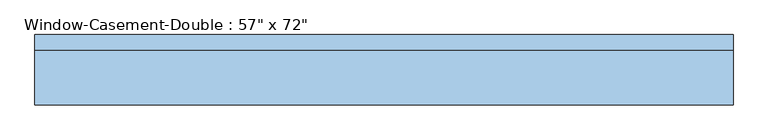
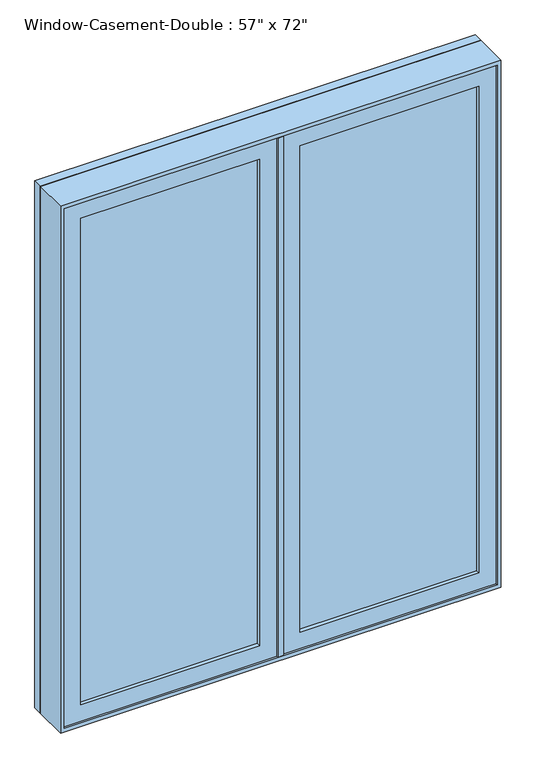
"""IFC4 building model written with IfcOpenShell, lengths in millimetres: window geometry."""

from ifc_helpers import new_model, si_unit, frame, origin, place, context, project, spatial, polyline, outline, extrude, faceted_brep, source, transform, mapped, element, save


def window_01a3843f(model_context):
    return source(origin(), model_context, "Body", "SolidModel", [
        faceted_brep([(9.525, -82.55, 2730.5), (9.525, -31.75, 2730.5), (-9.525, -31.75, 2730.5), (-9.525, -82.55, 2730.5), (9.525, -82.55, 927.1), (-9.525, -82.55, 927.1), (-9.525, -31.75, 927.1), (9.525, -31.75, 927.1), (-9.525, -31.75, 2711.45), (-9.525, -31.75, 946.15), (-30.1625, -31.75, 2711.45), (-30.1625, -31.75, 946.15), (-30.1625, 31.75, 2711.45), (-30.1625, 31.75, 946.15), (30.1625, 31.75, 2711.45), (30.1625, 31.75, 946.15), (30.1625, -31.75, 2711.45), (30.1625, -31.75, 946.15), (9.525, -31.75, 2711.45), (9.525, -31.75, 946.15)], [[[0, 1, 2, 3]], [[4, 5, 6, 7]], [[3, 5, 4, 0]], [[2, 8, 9, 6, 5, 3]], [[8, 10, 11, 9]], [[10, 12, 13, 11]], [[12, 14, 15, 13]], [[14, 16, 17, 15]], [[16, 18, 19, 17]], [[0, 4, 7, 19, 18, 1]], [[8, 2, 1, 18]], [[19, 7, 6, 9]], [[9, 11, 13, 15, 17, 19]], [[18, 16, 14, 12, 10, 8]]]),
        extrude(outline(polyline([(-66.675, -63.5), (-654.05, -63.5), (-654.05, -57.15), (-66.675, -57.15), (-66.675, -63.5)])), frame((0.0, 0.0, 984.25), z_axis=(0.0, 0.0, 1.0), x_axis=(1.0, 0.0, 0.0)), (0.0, 0.0, 1.0), 1689.1),
        extrude(outline(polyline([(-654.05, -44.45), (-66.675, -44.45), (-66.675, -50.8), (-654.05, -50.8), (-654.05, -44.45)])), frame((0.0, 0.0, 984.25), z_axis=(0.0, 0.0, 1.0), x_axis=(1.0, 0.0, 0.0)), (0.0, 0.0, 1.0), 1689.1),
        extrude(outline(polyline([(654.05, -63.5), (66.675, -63.5), (66.675, -57.15), (654.05, -57.15), (654.05, -63.5)])), frame((0.0, 0.0, 984.25), z_axis=(0.0, 0.0, 1.0), x_axis=(1.0, 0.0, 0.0)), (0.0, 0.0, 1.0), 1689.1),
        extrude(outline(polyline([(66.675, -44.45), (654.05, -44.45), (654.05, -50.8), (66.675, -50.8), (66.675, -44.45)])), frame((0.0, 0.0, 984.25), z_axis=(0.0, 0.0, 1.0), x_axis=(1.0, 0.0, 0.0)), (0.0, 0.0, 1.0), 1689.1),
        extrude(outline(polyline([(2730.5, -9.525), (2730.5, -711.2), (927.1, -711.2), (927.1, -9.525), (2730.5, -9.525)]), holes=[polyline([(2673.35, -654.05), (2673.35, -66.675), (984.25, -66.675), (984.25, -654.05), (2673.35, -654.05)])]), frame((0.0, -76.2, 0.0), z_axis=(0.0, 1.0, 0.0), x_axis=(0.0, 0.0, 1.0)), (0.0, 0.0, 1.0), 44.45),
        extrude(outline(polyline([(927.1, 9.525), (927.1, 711.2), (2730.5, 711.2), (2730.5, 9.525), (927.1, 9.525)]), holes=[polyline([(984.25, 654.05), (984.25, 66.675), (2673.35, 66.675), (2673.35, 654.05), (984.25, 654.05)])]), frame((0.0, -76.2, 0.0), z_axis=(0.0, 1.0, 0.0), x_axis=(0.0, 0.0, 1.0)), (0.0, 0.0, 1.0), 44.45),
        extrude(outline(polyline([(2743.2, -723.9), (914.4, -723.9), (914.4, 723.9), (2743.2, 723.9), (2743.2, -723.9)]), holes=[polyline([(2724.15, 704.85), (933.45, 704.85), (933.45, -704.85), (2724.15, -704.85), (2724.15, 704.85)])]), frame((0.0, 31.75, 0.0), z_axis=(0.0, 1.0, 0.0), x_axis=(0.0, 0.0, 1.0)), (0.0, 0.0, 1.0), 31.75),
        faceted_brep([(692.15, -31.75, 2711.45), (-692.15, -31.75, 2711.45), (-692.15, 31.75, 2711.45), (692.15, 31.75, 2711.45), (711.2, -82.55, 2730.5), (-711.2, -82.55, 2730.5), (-711.2, -31.75, 2730.5), (711.2, -31.75, 2730.5), (723.9, 31.75, 2743.2), (-723.9, 31.75, 2743.2), (-723.9, -82.55, 2743.2), (723.9, -82.55, 2743.2), (-692.15, -31.75, 946.15), (-692.15, 31.75, 946.15), (-711.2, -82.55, 927.1), (-711.2, -31.75, 927.1), (-723.9, 31.75, 914.4), (-723.9, -82.55, 914.4), (692.15, -31.75, 946.15), (692.15, 31.75, 946.15), (711.2, -82.55, 927.1), (711.2, -31.75, 927.1), (723.9, 31.75, 914.4), (723.9, -82.55, 914.4)], [[[0, 1, 2, 3]], [[4, 5, 6, 7]], [[8, 9, 10, 11]], [[1, 12, 13, 2]], [[5, 14, 15, 6]], [[9, 16, 17, 10]], [[12, 18, 19, 13]], [[14, 20, 21, 15]], [[16, 22, 23, 17]], [[9, 8, 22, 16], [3, 2, 13, 19]], [[18, 0, 3, 19]], [[7, 6, 15, 21], [1, 0, 18, 12]], [[20, 4, 7, 21]], [[22, 8, 11, 23]], [[11, 10, 17, 23], [5, 4, 20, 14]]]),
    ])


if __name__ == "__main__":
    model = new_model("IFC4")
    model_context = context("Model", 3, world=origin())
    ifc_project = project(units=[si_unit("LENGTHUNIT", "METRE", prefix="MILLI")], contexts=[model_context])
    site = spatial("IfcSite", under=ifc_project)
    building = spatial("IfcBuilding", under=site)
    placement = place(None, origin())
    window_shape = window_01a3843f(model_context)
    element("IfcWindow", 1, ObjectType="Window-Casement-Double : 57\" x 72\"", at=placement, inside=building, context=model_context, shape_type="MappedRepresentation", body=[
        mapped(window_shape, transform((0.0, 0.0, 0.0), x_axis=(1.0, 0.0, 0.0), y_axis=(0.0, 1.0, 0.0), z_axis=(0.0, 0.0, 1.0))),
    ])
    save(model, "model.ifc")

# Revit data of these elements
# Type "Window-Casement-Double : 57\" x 72\""
#   Type Mark = "17"
#   Fire Rating = "0.5h"
#   Assembly Code = "B2020100"
#   Analytic Construction = "Double glazing - domestic"
#   Frame Extension [instance default] = 0' - 0 1/4"
#   Window Inset [instance default] = 0' - 0"
#   Wall Thickness [instance default] = 0' - 6"
#   Interior Wall Closure [instance default] = 0' - 2 1/4"
#   Half Width = 2' - 4 1/2"
#   Visual Light Transmittance = 0.81
#   Thermal Resistance (R) = 1.8146 (h·ft²·°F)/BTU
#   Solar Heat Gain Coefficient = 0.76
#   Rough Width = 4' - 9 1/2"
#   Rough Height = 6' - 0 1/2"
#   Height = 6' - 0"
#   Heat Transfer Coefficient (U) = 0.5511 BTU/(h·ft²·°F)
#   Exterior Wall Closure [instance default] = 0' - 1 1/4"
#   Extension Jamb [instance default] = 0' - 2 1/4"
#   Default Sill Height = 3' - 0"
#   Width = 4' - 9"
#   Define Thermal Properties by = 0
#   Muntin Visibility = yes
#   Interior Trim Visibility [instance default] = yes
#   Exterior Trim Visibility [instance default] = yes
#   Extension Jamb Visibility [instance default] = yes
#   Interior Trim Material = Wood - Stained
#   Muntin Pattern = Muntin Pattern_2x2 : Muntin Pattern_2x2
#   Interior Trim = Trim-Window-Interior-Flat : Picture Frame
#   Interior Frame Material = Wood - Stained
#   Glass Panel Material = Glass
#   Exterior Trim Material = Clad - White
#   Exterior Trim = Trim-Window-Exterior-Flat : with Sill
#   Exterior Frame Material = Clad - White
#   Wall Closure = (empty or 0)
# Element 1 (IfcWindow, "Window-Casement-Double : 57\" x 72\"")
#   Wall Thickness = 0' - 5"
#   Extension Jamb = 0' - 1 1/4"
#   Materials on its faces: "Wood - Stained", "Glass", "Clad - White"
# Materials
#   "Wood - Stained": class "Wood", colour RGB 224 178 126, transparency 0, Cost = 0
#   "Glass": class "Glass", colour RGB 0 128 192, transparency 0.75, Description = "Soda Lime Glass", Cost = 0
#   "Clad - White": class "Wood", colour RGB 242 242 238, transparency 0, Cost = 0
